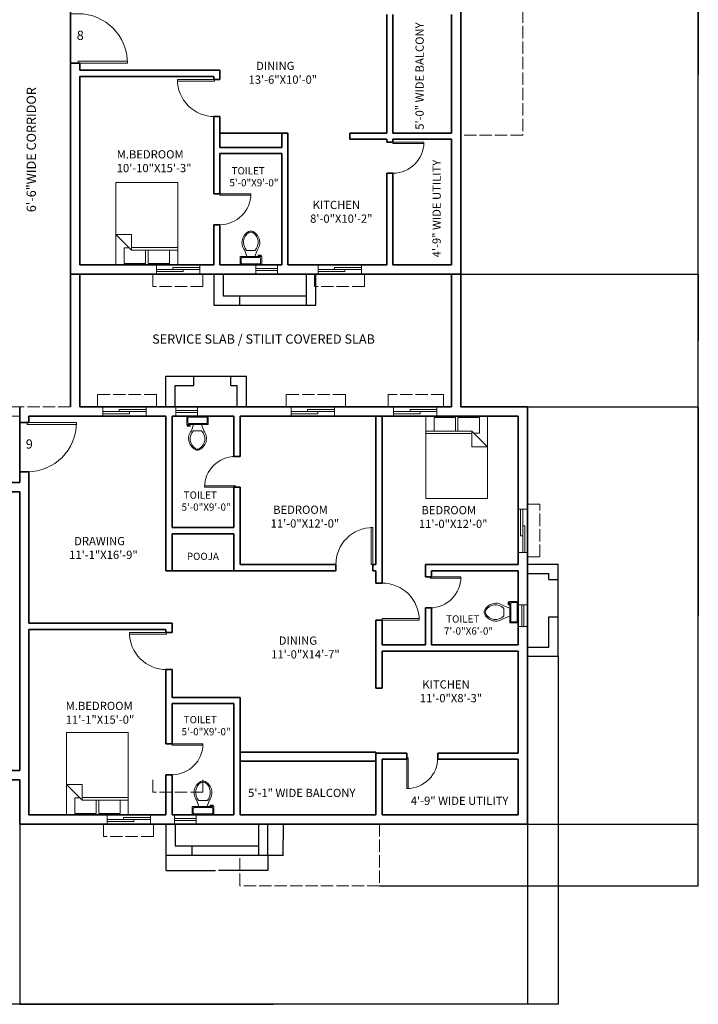
# Model space of a CAD drawing. Units: inches. Extents: x -69 to 2453, y 4803 to 7122.
# Tile 6 of 9: x 1794 to 2453, y 4803 to 5759. Entities that reach past the tile are written whole.
import ezdxf

# ---------------------------------------------------------------- set-up
doc = ezdxf.new("R2010")
doc.units = ezdxf.units.IN
doc.linetypes.add('ACAD_ISO02W100', pattern=[15, 12, -3])
for name, color, linetype, lineweight in [('A-ANNO-DIMS', 2, 'Continuous', 18), ('A-ANNO-IDEN', 2, 'Continuous', 18), ('A-AREA-IDEN', 7, 'Continuous', 18), ('A-DOOR', 3, 'Continuous', 18), ('A-FLOR-FIXT', 9, 'Continuous', 18), ('A-FLOR-OVHD', 8, 'ACAD_ISO02W100', 13), ('A-FURN', 8, 'Continuous', 18), ('A-GLAZ', 244, 'Continuous', 18), ('A-WALL', 7, 'Continuous', 35), ('A-WALL-SRVC', 7, 'Continuous', 30)]:
    doc.layers.add(name, color=color, linetype=linetype, lineweight=lineweight)
doc.styles.get("Standard").update_dxf_attribs({"font": 'arial.ttf'})
doc.dimstyles.get("Standard").update_dxf_attribs({"dimtxt": 0.18, "dimasz": 0.18, "dimexe": 0.18, "dimexo": 0.0625, "dimgap": 0.09, "dimtad": 0, "dimtih": 1, "dimtoh": 1, "dimdec": 4, "dimzin": 0, "dimdsep": 46, "dimtxsty": 'Standard', "dimcen": 0.09, "dimadec": 0, "dimazin": 0, "dimtfac": 1, "dimtdec": 4, "dimtofl": 0, "dimtmove": 0, "dimatfit": 3, "dimfxl": 1, "dimtolj": 1, "dimtzin": 0, "dimarcsym": 0})

# ---------------------------------------------------------------- blocks, each defined once
blk = doc.blocks.new('*U12')
for p, q in [((-40, 0), (-40, -6)), ((0, 0), (0, -6))]:
    blk.add_line(p, q)
blk.add_lwpolyline([(0, 0), (0, 40), (-1.75, 40), (-1.75, 0)], close=True)
blk.add_arc((0, 0), 40, 90, 180)
blk = doc.blocks.new('*U20')
for p, q in [((0, 0), (0, -6)), ((40, 0), (40, -6))]:
    blk.add_line(p, q)
blk.add_lwpolyline([(0, 0), (0, 40), (1.75, 40), (1.75, 0)], close=True)
blk.add_arc((0, 0), 40, 0, 90)
blk = doc.blocks.new('*U13')
for p, q in [((0, 0), (0, -6)), ((40, 0), (40, -6))]:
    blk.add_line(p, q)
blk.add_lwpolyline([(0, 0), (0, 40), (1.75, 40), (1.75, 0)], close=True)
blk.add_arc((0, 0), 40, 0, 90)
blk = doc.blocks.new('*U11')
for p, q in [((-40, 0), (-40, 6)), ((0, 0), (0, 6))]:
    blk.add_line(p, q)
blk.add_lwpolyline([(0, 0), (0, -40), (-1.75, -40), (-1.75, 0)], close=True)
blk.add_arc((0, 0), 40, 180, 270)
blk = doc.blocks.new('*U17')
for p, q in [((0, 0), (0, 6)), ((40, 0), (40, 6))]:
    blk.add_line(p, q)
blk.add_lwpolyline([(0, 0), (0, -40), (1.75, -40), (1.75, 0)], close=True)
blk.add_arc((0, 0), 40, 270, 0)
blk = doc.blocks.new('*U18')
for p, q in [((0, 0), (0, -6)), ((-40, 0), (-40, -6))]:
    blk.add_line(p, q)
blk.add_lwpolyline([(0, 0), (0, 40), (-1.75, 40), (-1.75, 0)], close=True)
blk.add_arc((0, 0), 40, 90, 180)
blk = doc.blocks.new('*U19')
for p, q in [((0, 0), (0, -6)), ((-40, 0), (-40, -6))]:
    blk.add_line(p, q)
blk.add_lwpolyline([(0, 0), (0, 40), (-1.75, 40), (-1.75, 0)], close=True)
blk.add_arc((0, 0), 40, 90, 180)
blk = doc.blocks.new('*U14')
for p, q in [((0, 0), (0, -6)), ((-40, 0), (-40, -6))]:
    blk.add_line(p, q)
blk.add_lwpolyline([(0, 0), (0, 40), (-1.75, 40), (-1.75, 0)], close=True)
blk.add_arc((0, 0), 40, 90, 180)
blk = doc.blocks.new('Bed - Queen')
for p, q in [((0, -80.00003), (0, 0)), ((0, 0), (59.99999, 0)), ((59.99999, 0), (59.99999, -80.00003)), ((7.99999, -1.2), (28.79998, -1.2)), ((7.99999, -14.4), (7.99999, -1.2)), ((28.79998, -1.2), (28.79998, -14.4)), ((31.19999, -1.2), (51.99999, -1.2)), ((31.19999, -14.4), (31.19999, -1.2)), ((51.99999, -1.2), (51.99999, -16.4)), ((0, -14.4), (44.8, -14.4)), ((44.8, -16.8), (0, -16.8)), ((59.99999, -29.6), (44.8, -14.4)), ((44.8, -14.4), (44.8, -29.6)), ((51.99999, -16.4), (46.79936, -16.4)), ((44.8, -29.6), (59.99999, -29.6)), ((59.99999, -80.00003), (0, -80.00003))]:
    blk.add_line(p, q)
blk = doc.blocks.new('*U33')
for p, q in [((-10, -8.5), (-8, -8.5)), ((-10, -9.5), (-10, -8.5)), ((-7, -9.5), (-10, -9.5)), ((-8, -8.5), (-8, -8)), ((-7, -8), (-7, -9.5)), ((-4, -8), (-6, -14)), ((4, -8), (6, -14)), ((9.5, -6), (9.5, -2)), ((4, -14), (-4, -14))]:
    blk.add_line(p, q)
blk.add_lwpolyline([(10.5, -8), (10.5, 0), (-10.5, 0), (-10.5, -8)], close=True)
for points in [[(-9.5, -2), (-9.5, -6)], [(8.5, -1), (-8.5, -1)], [(-8.5, -7), (8.5, -7)]]:
    blk.add_lwpolyline(points)
for centre, radius, start, end in [((-8.62, -1.88), 0.884, 81.8699, 188.1301), ((-8.62, -6.12), 0.884, 171.8699, 278.1301), ((8.62, -1.88), 0.884, 351.8699, 98.1301), ((8.62, -6.12), 0.884, 261.8699, 8.1301), ((3.52, -21.58), 12.17, 141.46911, 247.97143), ((4.2, -21.82), 11.33, 136.36773, 238.94682), ((-3.52, -21.58), 12.17, 292.02843, 38.53071), ((-4.2, -21.82), 11.33, 301.05301, 43.63209), ((0, -27.88), 4, 245.73182, 294.26817), ((0, -29), 4, 254.86053, 285.13947)]:
    blk.add_arc(centre, radius, start, end)
blk = doc.blocks.new('WINDOW-VENT-21IN')
for p, q in [((0, 5.5), (21, 5.5)), ((0, 3.5), (21, 3.5))]:
    blk.add_line(p, q)
blk.add_lwpolyline([(0, 9), (21, 9), (21, 0), (0, 0)], close=True)
blk = doc.blocks.new('WINDOW-SLIDING-42IN')
for p, q in [((2.5, 42), (2.5, 16)), ((4.5, 42), (4.5, 0)), ((4.5, 26), (6.5, 26)), ((6.5, 26), (6.5, 0)), ((4.5, 16), (2.5, 16))]:
    blk.add_line(p, q)
blk.add_lwpolyline([(0, 42), (9, 42), (9, 0), (0, 0)], close=True)
blk = doc.blocks.new('SUNSHADE-48IN')
for p, q in [((0, 0), (0, 12)), ((48.4, 12), (48.4, 0)), ((48.4, 0), (0, 0))]:
    blk.add_line(p, q)
blk = doc.blocks.new('SUNSHADE-57IN')
for p, q in [((57.14, 12), (0, 12)), ((0, 12), (0, 0)), ((57.14, 0), (57.14, 12))]:
    blk.add_line(p, q)
blk = doc.blocks.new('SUNSHADE-51IN')
for p, q in [((12, 51.36), (0, 51.36)), ((12, 0), (12, 51.36)), ((0, 0), (12, 0))]:
    blk.add_line(p, q)
blk = doc.blocks.new('SERVICE-BAY-78IN')
for p, q in [((0, 30), (78.14, 30)), ((0, 0), (0, 30)), ((27.07, 21), (27.07, 30)), ((63.07, 21), (63.07, 30)), ((78.14, 0), (78.14, 30)), ((9, 0), (9, 21)), ((9, 21), (27.07, 21)), ((63.07, 21), (69.14, 21)), ((69.14, 0), (69.14, 21))]:
    blk.add_line(p, q)
blk = doc.blocks.new('SERVICE-BAY-99IN')
for p, q in [((0, 30), (0, 0)), ((9, 30), (9, 9)), ((90.11, 0), (90.11, 30)), ((99.11, 0), (99.11, 30)), ((0, 0), (99.11, 0)), ((9, 9), (90.11, 9)), ((25.44, 0), (25.44, 9))]:
    blk.add_line(p, q)
blk = doc.blocks.new('*D67')
at = {"layer": 'A-ANNO-DIMS', "color": 0, "lineweight": -2, "transparency": 16777216}
for p, q in [((1935.51, 4947.65), (1935.51, 4932.67)), ((2034.62, 4947.65), (2034.62, 4932.67)), ((1935.69, 4932.85), (1983.66, 4932.85)), ((2034.44, 4932.85), (1986.47, 4932.85))]:
    blk.add_line(p, q, dxfattribs=at)
at = {"layer": 'A-ANNO-DIMS', "color": 0, "transparency": 16777216}
for points in [[(1935.69, 4932.88), (1935.69, 4932.82), (1935.51, 4932.85)], [(2034.44, 4932.88), (2034.44, 4932.82), (2034.62, 4932.85)]]:
    blk.add_solid(points, dxfattribs=at)
at = {"layer": 'Defpoints', "color": 0, "transparency": 16777216}
for p in [(1935.51, 4947.72), (2034.62, 4947.72), (2034.62, 4932.85)]:
    blk.add_point(p, dxfattribs=at)
at = {"layer": 'A-ANNO-DIMS', "color": 0, "transparency": 16777216, "insert": (1985.06, 4932.85), "char_height": 0.18, "attachment_point": 5}
blk.add_mtext('\\A1;SERVICE BAY 99 TYP.', dxfattribs=at)
blk = doc.blocks.new('*D68')
at = {"layer": 'A-ANNO-DIMS', "color": 0, "lineweight": -2, "transparency": 16777216}
for p, q in [((2034.68, 4977.72), (2049.67, 4977.72)), ((2049.49, 4977.54), (2049.49, 4962.9)), ((2049.49, 4947.9), (2049.49, 4962.53)), ((2034.68, 4947.72), (2049.67, 4947.72))]:
    blk.add_line(p, q, dxfattribs=at)
at = {"layer": 'A-ANNO-DIMS', "color": 0, "transparency": 16777216}
for points in [[(2049.46, 4977.54), (2049.52, 4977.54), (2049.49, 4977.72)], [(2049.46, 4947.9), (2049.52, 4947.9), (2049.49, 4947.72)]]:
    blk.add_solid(points, dxfattribs=at)
at = {"layer": 'Defpoints', "color": 0, "transparency": 16777216}
for p in [(2034.62, 4977.72), (2049.49, 4977.72), (2034.62, 4947.72)]:
    blk.add_point(p, dxfattribs=at)
at = {"layer": 'A-ANNO-DIMS', "color": 0, "transparency": 16777216, "insert": (2049.49, 4962.72), "char_height": 0.18, "attachment_point": 5}
blk.add_mtext('\\A1;30 TYP.', dxfattribs=at)
blk = doc.blocks.new('*D86')
at = {"layer": 'A-ANNO-DIMS', "color": 0, "lineweight": -2, "transparency": 16777216}
for p, q in [((1673.51, 5020.65), (1673.51, 4802.79)), ((1793.51, 5020.65), (1793.51, 4802.79)), ((1673.69, 4802.97), (1733.23, 4802.97)), ((1793.33, 4802.97), (1733.79, 4802.97))]:
    blk.add_line(p, q, dxfattribs=at)
at = {"layer": 'A-ANNO-DIMS', "color": 0, "transparency": 16777216}
for points in [[(1673.69, 4803), (1673.69, 4802.94), (1673.51, 4802.97)], [(1793.33, 4803), (1793.33, 4802.94), (1793.51, 4802.97)]]:
    blk.add_solid(points, dxfattribs=at)
at = {"layer": 'Defpoints', "color": 0, "transparency": 16777216}
for p in [(1673.51, 5020.72), (1793.51, 5020.72), (1793.51, 4802.97)]:
    blk.add_point(p, dxfattribs=at)
at = {"layer": 'A-ANNO-DIMS', "color": 0, "transparency": 16777216, "insert": (1733.51, 4802.97), "char_height": 0.18, "attachment_point": 5}
blk.add_mtext('\\A1;120', dxfattribs=at)
blk = doc.blocks.new('*D87')
at = {"layer": 'A-ANNO-DIMS', "color": 0, "lineweight": -2, "transparency": 16777216}
for p, q in [((1793.51, 4977.65), (1793.51, 4802.79)), ((2286.51, 4977.65), (2286.51, 4802.79)), ((1793.69, 4802.97), (2039.72, 4802.97)), ((2286.33, 4802.97), (2040.3, 4802.97))]:
    blk.add_line(p, q, dxfattribs=at)
at = {"layer": 'A-ANNO-DIMS', "color": 0, "transparency": 16777216}
for points in [[(1793.69, 4803), (1793.69, 4802.94), (1793.51, 4802.97)], [(2286.33, 4803), (2286.33, 4802.94), (2286.51, 4802.97)]]:
    blk.add_solid(points, dxfattribs=at)
at = {"layer": 'Defpoints', "color": 0, "transparency": 16777216}
for p in [(1793.51, 4977.72), (2286.51, 4977.72), (2286.51, 4802.97)]:
    blk.add_point(p, dxfattribs=at)
at = {"layer": 'A-ANNO-DIMS', "color": 0, "transparency": 16777216, "insert": (2040.01, 4802.97), "char_height": 0.18, "attachment_point": 5}
blk.add_mtext('\\A1;493', dxfattribs=at)
blk = doc.blocks.new('*D88')
at = {"layer": 'A-ANNO-DIMS', "color": 0, "lineweight": -2, "transparency": 16777216}
for p, q in [((2286.57, 5382.72), (2452.44, 5382.72)), ((2452.26, 5382.54), (2452.26, 5180.4)), ((2452.26, 4977.9), (2452.26, 5180.03)), ((2286.57, 4977.72), (2452.44, 4977.72))]:
    blk.add_line(p, q, dxfattribs=at)
at = {"layer": 'A-ANNO-DIMS', "color": 0, "transparency": 16777216}
for points in [[(2452.23, 5382.54), (2452.29, 5382.54), (2452.26, 5382.72)], [(2452.23, 4977.9), (2452.29, 4977.9), (2452.26, 4977.72)]]:
    blk.add_solid(points, dxfattribs=at)
at = {"layer": 'Defpoints', "color": 0, "transparency": 16777216}
for p in [(2286.51, 5382.72), (2452.26, 5382.72), (2286.51, 4977.72)]:
    blk.add_point(p, dxfattribs=at)
at = {"layer": 'A-ANNO-DIMS', "color": 0, "transparency": 16777216, "insert": (2452.26, 5180.22), "char_height": 0.18, "attachment_point": 5}
blk.add_mtext('\\A1;405', dxfattribs=at)
blk = doc.blocks.new('*D89')
at = {"layer": 'A-ANNO-DIMS', "color": 0, "lineweight": -2, "transparency": 16777216}
for p, q in [((2222.07, 5511.72), (2452.44, 5511.72)), ((2452.26, 5511.54), (2452.26, 5447.4)), ((2452.26, 5382.9), (2452.26, 5447.03)), ((2222.07, 5382.72), (2452.44, 5382.72))]:
    blk.add_line(p, q, dxfattribs=at)
at = {"layer": 'A-ANNO-DIMS', "color": 0, "transparency": 16777216}
for points in [[(2452.23, 5511.54), (2452.29, 5511.54), (2452.26, 5511.72)], [(2452.23, 5382.9), (2452.29, 5382.9), (2452.26, 5382.72)]]:
    blk.add_solid(points, dxfattribs=at)
at = {"layer": 'Defpoints', "color": 0, "transparency": 16777216}
for p in [(2222.01, 5511.72), (2452.26, 5511.72), (2222.01, 5382.72)]:
    blk.add_point(p, dxfattribs=at)
at = {"layer": 'A-ANNO-DIMS', "color": 0, "transparency": 16777216, "insert": (2452.26, 5447.22), "char_height": 0.18, "attachment_point": 5}
blk.add_mtext('\\A1;129', dxfattribs=at)
blk = doc.blocks.new('*D90')
at = {"layer": 'A-ANNO-DIMS', "color": 0, "lineweight": -2, "transparency": 16777216}
for p, q in [((2222.07, 5898.72), (2452.44, 5898.72)), ((2452.26, 5898.54), (2452.26, 5705.4)), ((2452.26, 5511.9), (2452.26, 5705.03)), ((2222.07, 5511.72), (2452.44, 5511.72))]:
    blk.add_line(p, q, dxfattribs=at)
at = {"layer": 'A-ANNO-DIMS', "color": 0, "transparency": 16777216}
for points in [[(2452.23, 5898.54), (2452.29, 5898.54), (2452.26, 5898.72)], [(2452.23, 5511.9), (2452.29, 5511.9), (2452.26, 5511.72)]]:
    blk.add_solid(points, dxfattribs=at)
at = {"layer": 'Defpoints', "color": 0, "transparency": 16777216}
for p in [(2222.01, 5898.72), (2452.26, 5898.72), (2222.01, 5511.72)]:
    blk.add_point(p, dxfattribs=at)
at = {"layer": 'A-ANNO-DIMS', "color": 0, "transparency": 16777216, "insert": (2452.26, 5705.22), "char_height": 0.18, "attachment_point": 5}
blk.add_mtext('\\A1;387', dxfattribs=at)
blk = doc.blocks.new('*D95')
at = {"layer": 'A-ANNO-DIMS', "color": 0, "lineweight": -2, "transparency": 16777216}
for p, q in [((96.509262, 5020.652777), (96.509262, 4802.785277)), ((2286.509262, 4977.652777), (2286.509262, 4802.785277)), ((96.689262, 4802.965277), (1191.149262, 4802.965277)), ((2286.329262, 4802.965277), (1191.869262, 4802.965277))]:
    blk.add_line(p, q, dxfattribs=at)
at = {"layer": 'A-ANNO-DIMS', "color": 0, "transparency": 16777216}
for points in [[(96.689262, 4802.995277), (96.689262, 4802.935277), (96.509262, 4802.965277)], [(2286.329262, 4802.995277), (2286.329262, 4802.935277), (2286.509262, 4802.965277)]]:
    blk.add_solid(points, dxfattribs=at)
at = {"layer": 'Defpoints', "color": 0, "transparency": 16777216}
for p in [(96.509262, 5020.715277), (2286.509262, 4977.715277), (2286.509262, 4802.965277)]:
    blk.add_point(p, dxfattribs=at)
at = {"layer": 'A-ANNO-DIMS', "color": 0, "transparency": 16777216, "insert": (1191.509262, 4802.965277), "char_height": 0.18, "attachment_point": 5}
blk.add_mtext('\\A1;2190', dxfattribs=at)
blk = doc.blocks.new('*D96')
at = {"layer": 'A-ANNO-DIMS', "color": 0, "lineweight": -2, "transparency": 16777216}
for p, q in [((2044.63, 7006.72), (2452.44, 7006.72)), ((2452.26, 7006.54), (2452.26, 5962.4)), ((2452.26, 4917.9), (2452.26, 5962.03)), ((2143.12, 4917.72), (2452.44, 4917.72))]:
    blk.add_line(p, q, dxfattribs=at)
at = {"layer": 'A-ANNO-DIMS', "color": 0, "transparency": 16777216}
for points in [[(2452.23, 7006.54), (2452.29, 7006.54), (2452.26, 7006.72)], [(2452.23, 4917.9), (2452.29, 4917.9), (2452.26, 4917.72)]]:
    blk.add_solid(points, dxfattribs=at)
at = {"layer": 'Defpoints', "color": 0, "transparency": 16777216}
for p in [(2044.57, 7006.72), (2452.26, 7006.72), (2143.06, 4917.72)]:
    blk.add_point(p, dxfattribs=at)
at = {"layer": 'A-ANNO-DIMS', "color": 0, "transparency": 16777216, "insert": (2452.26, 5962.22), "char_height": 0.18, "attachment_point": 5}
blk.add_mtext('\\A1;2089', dxfattribs=at)
blk = doc.blocks.new('*D105')
at = {"layer": 'A-ANNO-DIMS', "color": 0, "lineweight": -2, "transparency": 16777216}
for p, q in [((66.509262, 5170.610035), (66.509262, 4802.785277)), ((2316.509262, 5140.587945), (2316.509262, 4802.785277)), ((66.689262, 4802.965277), (1191.149262, 4802.965277)), ((2316.329262, 4802.965277), (1191.869262, 4802.965277))]:
    blk.add_line(p, q, dxfattribs=at)
at = {"layer": 'A-ANNO-DIMS', "color": 0, "transparency": 16777216}
for points in [[(66.689262, 4802.995277), (66.689262, 4802.935277), (66.509262, 4802.965277)], [(2316.329262, 4802.995277), (2316.329262, 4802.935277), (2316.509262, 4802.965277)]]:
    blk.add_solid(points, dxfattribs=at)
at = {"layer": 'Defpoints', "color": 0, "transparency": 16777216}
for p in [(66.509262, 5170.672535), (2316.509262, 5140.650445), (2316.509262, 4802.965277)]:
    blk.add_point(p, dxfattribs=at)
at = {"layer": 'A-ANNO-DIMS', "color": 0, "transparency": 16777216, "insert": (1191.509262, 4802.965277), "char_height": 0.18, "attachment_point": 5}
blk.add_mtext('\\A1;2250', dxfattribs=at)

msp = doc.modelspace()

# ---------------------------------------------------------------- linework, layer by layer
at = {"layer": 'A-FLOR-OVHD'}
for p, q in [((2282.01, 5767.63), (2282.01, 5646.75)), ((2282.01, 5646.75), (2222.01, 5646.75)), ((2109.75, 5394.72), (2052.22, 5394.72)), ((2052.22, 5394.72), (2052.22, 5382.72)), ((2109.75, 5382.72), (2109.75, 5394.72)), ((2204.95, 5394.72), (2151.19, 5394.72)), ((2151.19, 5394.72), (2151.19, 5382.72)), ((2204.95, 5382.72), (2204.95, 5394.72)), ((1843.01, 5382.72), (1673.51, 5382.72)), ((1793.51, 5373.72), (1673.51, 5373.72)), ((2143.06, 4977.72), (2143.06, 4917.72)), ((2007.19, 4917.72), (2007.19, 4947.72)), ((2143.06, 4917.72), (2007.19, 4917.72))]:
    msp.add_line(p, q, dxfattribs=at)
at = {"layer": 'A-WALL'}
for p, q in [((2222.01, 6543.72), (2222.01, 5382.72)), ((1843.01, 6308.22), (1843.01, 5382.72)), ((2150.01, 5763.72), (2150.01, 5648.72)), ((2156.01, 5763.72), (2156.01, 5648.72)), ((2213.01, 5763.72), (2213.01, 5648.72)), ((1852.01, 5716.52), (1843.01, 5716.52)), ((1852.01, 5716.52), (1852.01, 5709.72)), ((1852.01, 5709.72), (1988.01, 5709.72)), ((1988.01, 5709.72), (1988.01, 5700.72)), ((1852.01, 5703.72), (1982.01, 5703.72)), ((1852.01, 5703.72), (1852.01, 5520.72)), ((1982.01, 5703.72), (1982.01, 5700.72)), ((1982.01, 5700.72), (1988.01, 5700.72)), ((1982.01, 5664.72), (1988.01, 5664.72)), ((1982.01, 5664.72), (1982.01, 5589.72)), ((1988.01, 5664.72), (1988.01, 5634.72)), ((1988.01, 5648.72), (2054.01, 5648.72)), ((2048.01, 5648.72), (2048.01, 5634.72)), ((2054.01, 5648.72), (2054.01, 5520.72)), ((2114.01, 5648.72), (2114.01, 5642.72)), ((2114.01, 5648.72), (2150.01, 5648.72)), ((2150.01, 5642.72), (2114.01, 5642.72)), ((2150.01, 5642.72), (2150.01, 5639.72)), ((2156.01, 5648.72), (2213.01, 5648.72)), ((2156.01, 5642.72), (2156.01, 5639.72)), ((2156.01, 5642.72), (2213.01, 5642.72)), ((2213.01, 5642.72), (2213.01, 5520.72)), ((1988.01, 5634.72), (2048.01, 5634.72)), ((2150.01, 5639.72), (2156.01, 5639.72)), ((1988.01, 5628.72), (2048.01, 5628.72)), ((1988.01, 5628.72), (1988.01, 5589.72)), ((2048.01, 5628.72), (2048.01, 5520.72)), ((2150.01, 5609.72), (2156.01, 5609.72)), ((2150.01, 5609.72), (2150.01, 5520.72)), ((2156.01, 5609.72), (2156.01, 5520.72)), ((1988.01, 5589.72), (1982.01, 5589.72)), ((1988.01, 5559.72), (1982.01, 5559.72)), ((1982.01, 5559.72), (1982.01, 5520.72)), ((1988.01, 5559.72), (1988.01, 5520.72)), ((1852.01, 5520.72), (1982.01, 5520.72)), ((1988.01, 5520.72), (2048.01, 5520.72)), ((2054.01, 5520.72), (2150.01, 5520.72)), ((2156.01, 5520.72), (2213.01, 5520.72)), ((1843.01, 5511.72), (2222.01, 5511.72)), ((1852.01, 5511.72), (1852.01, 5382.72)), ((2213.01, 5511.72), (2213.01, 5382.72)), ((1793.51, 5382.72), (1793.51, 5309.33)), ((1852.01, 5382.72), (2213.01, 5382.72)), ((2222.01, 5382.72), (2286.51, 5382.72)), ((2286.51, 5382.72), (2286.51, 4977.72)), ((1802.51, 5373.72), (1935.51, 5373.72)), ((1802.51, 5373.72), (1802.51, 5367.72)), ((1935.51, 5373.72), (1935.51, 5223.72)), ((1941.51, 5373.72), (1941.51, 5265.72)), ((1941.51, 5373.72), (2001.51, 5373.72)), ((2001.51, 5373.72), (2001.51, 5334.72)), ((2007.51, 5373.72), (2007.51, 5334.72)), ((2007.51, 5373.72), (2277.51, 5373.72)), ((2139.51, 5373.72), (2139.51, 5229.72)), ((2145.51, 5373.72), (2145.51, 5211.72)), ((2277.51, 5373.72), (2277.51, 5229.72)), ((1802.51, 5367.72), (1793.51, 5367.72)), ((2001.51, 5334.72), (2007.51, 5334.72)), ((1802.51, 5319.72), (1793.51, 5319.72)), ((1802.51, 5319.72), (1802.51, 5172.72)), ((1673.51, 5309.33), (1793.51, 5309.33)), ((1673.51, 5300.33), (1793.51, 5300.33)), ((1793.51, 5300.33), (1793.51, 5029.72)), ((2001.51, 5304.72), (2007.51, 5304.72)), ((2001.51, 5304.72), (2001.51, 5265.72)), ((2007.51, 5304.72), (2007.51, 5229.72)), ((1941.51, 5265.72), (2001.51, 5265.72)), ((1941.51, 5259.72), (2001.51, 5259.72)), ((1941.51, 5259.72), (1941.51, 5223.72)), ((2001.51, 5259.72), (2001.51, 5223.72)), ((2007.51, 5229.72), (2100.51, 5229.72)), ((2100.51, 5223.72), (2100.51, 5229.72)), ((2136.51, 5223.72), (2136.51, 5229.72)), ((2136.51, 5229.72), (2139.51, 5229.72)), ((2187.51, 5229.72), (2277.51, 5229.72)), ((2187.51, 5229.72), (2187.51, 5217.72)), ((1935.51, 5223.72), (2100.51, 5223.72)), ((2136.51, 5223.72), (2139.51, 5223.72)), ((2139.51, 5223.72), (2139.51, 5211.72)), ((2193.51, 5223.72), (2277.51, 5223.72)), ((2193.51, 5223.72), (2193.51, 5217.72)), ((2277.51, 5223.72), (2277.51, 5151.72)), ((2145.51, 5211.72), (2139.51, 5211.72)), ((2193.51, 5217.72), (2187.51, 5217.72)), ((2193.51, 5187.72), (2187.51, 5187.72)), ((2187.51, 5187.72), (2187.51, 5151.72)), ((2193.51, 5187.72), (2193.51, 5151.72)), ((1802.51, 5172.72), (1941.51, 5172.72)), ((1941.51, 5172.72), (1941.51, 5163.72)), ((2145.51, 5175.72), (2139.51, 5175.72)), ((2139.51, 5175.72), (2139.51, 5109.72)), ((2145.51, 5175.72), (2145.51, 5151.72)), ((1802.51, 5166.72), (1935.51, 5166.72)), ((1802.51, 5166.72), (1802.51, 4986.72)), ((1935.51, 5166.72), (1935.51, 5163.72)), ((1935.51, 5163.72), (1941.51, 5163.72)), ((2145.51, 5151.72), (2187.51, 5151.72)), ((2145.51, 5145.72), (2277.51, 5145.72)), ((2145.51, 5145.72), (2145.51, 5109.72)), ((2193.51, 5151.72), (2277.51, 5151.72)), ((2277.51, 5145.72), (2277.51, 5046.72)), ((1935.51, 5127.72), (1941.51, 5127.72)), ((1935.51, 5127.72), (1935.51, 5055.72)), ((1941.51, 5127.72), (1941.51, 5100.72)), ((2139.51, 5109.72), (2145.51, 5109.72)), ((1941.51, 5100.72), (2007.51, 5100.72)), ((2007.51, 5100.72), (2007.51, 4986.72)), ((1941.51, 5094.72), (2001.51, 5094.72)), ((1941.51, 5094.72), (1941.51, 5055.72)), ((2001.51, 5094.72), (2001.51, 4986.72)), ((1941.51, 5055.72), (1935.51, 5055.72)), ((2007.51, 5047.72), (2139.51, 5047.72)), ((2139.51, 5047.72), (2139.51, 4986.72)), ((2007.51, 5038.72), (2139.51, 5038.72)), ((2139.51, 5046.72), (2169.51, 5046.72)), ((2145.51, 5040.72), (2169.51, 5040.72)), ((2145.51, 5040.72), (2145.51, 4986.72)), ((2169.51, 5040.72), (2169.51, 5046.72)), ((2199.51, 5040.72), (2199.51, 5046.72)), ((2199.51, 5046.72), (2277.51, 5046.72)), ((2199.51, 5040.72), (2277.51, 5040.72)), ((2277.51, 5040.72), (2277.51, 4986.72)), ((1673.51, 5029.72), (1793.51, 5029.72)), ((354.66, 5020.72), (1793.51, 5020.72)), ((1793.51, 5020.72), (1793.51, 4977.72)), ((1941.51, 5025.72), (1935.51, 5025.72)), ((1935.51, 5025.72), (1935.51, 4986.72)), ((1941.51, 5025.72), (1941.51, 4986.72)), ((1802.51, 4986.72), (1935.51, 4986.72)), ((1941.51, 4986.72), (2001.51, 4986.72)), ((2007.51, 4986.72), (2139.51, 4986.72)), ((2145.51, 4986.72), (2277.51, 4986.72)), ((1793.51, 4977.72), (2286.51, 4977.72))]:
    msp.add_line(p, q, dxfattribs=at)
at = {"layer": 'A-WALL-SRVC'}
for p, q in [((2286.51, 5230.2), (2316.51, 5230.2)), ((2316.51, 5140.65), (2316.51, 5230.2)), ((2286.51, 5221.2), (2307.51, 5221.2)), ((2307.51, 5215.13), (2307.51, 5221.2)), ((2307.51, 5215.13), (2316.51, 5215.13)), ((2307.51, 5149.65), (2307.51, 5179.13)), ((2307.51, 5179.13), (2316.51, 5179.13)), ((2286.51, 5149.65), (2307.51, 5149.65)), ((2286.51, 5140.65), (2316.51, 5140.65))]:
    msp.add_line(p, q, dxfattribs=at)

# ---------------------------------------------------------------- block references
at = {"layer": 'A-DOOR'}
for name, p, xscale, yscale, zscale, rotation in [('*U12', (1850.21, 5716.52), 1.199999999999977, 1.199999999999977, 1.199999999999977, 270.0000000000001), ('*U17', (1982.61, 5700.72), 0.9, 0.9, 0.9, 270), ('*U13', (2156.01, 5639.72), 0.75, 0.75, 0.75, 270.0000000000001), ('*U13', (1988.01, 5589.72), 0.75, 0.75, 0.75, 270.0000000000001), ('*U20', (1800.71, 5367.72), 1.199999999999977, 1.199999999999977, 1.199999999999977, 270.0000000000001), ('*U11', (2003.01, 5304.72), 0.75, 0.75, 0.75, 270.0000000000001), ('*U18', (2145.51, 5175.72), 0.9, 0.9, 0.9, 270), ('*U13', (2192.01, 5217.72), 0.75, 0.75, 0.75, 270.0000000000001), ('*U17', (1936.11, 5163.72), 0.9, 0.9, 0.9, 270), ('*U13', (1941.51, 5055.72), 0.75, 0.75, 0.75, 270.0000000000001), ('*U14', (2169.51, 5042.22), 0.75, 0.75, 0.75, 180)]:
    msp.add_blockref(name, p, dxfattribs=dict(at, xscale=xscale, yscale=yscale, zscale=zscale, rotation=rotation))
at = {"layer": 'A-DOOR', "xscale": 0.9, "yscale": 0.9, "zscale": 0.9}
msp.add_blockref('*U19', (2136.51, 5229.72), dxfattribs=at)
at = {"layer": 'A-FLOR-FIXT'}
for p, rotation in [((2018.01, 5520.72), 180), ((2277.51, 5183.51), 270), ((1971.51, 4986.72), 180)]:
    msp.add_blockref('*U33', p, dxfattribs=dict(at, rotation=rotation))
msp.add_blockref('*U33', (1966.2, 5373.72), dxfattribs=at)
at = {"layer": 'A-FLOR-OVHD'}
for name, p in [('SUNSHADE-48IN', (1922.89, 5499.72)), ('SUNSHADE-48IN', (2079.86, 5499.72)), ('SUNSHADE-57IN', (1869.14, 5382.72)), ('SUNSHADE-51IN', (2286.51, 5237.15)), ('SUNSHADE-48IN', (1922.89, 5008.72)), ('SUNSHADE-48IN', (1874.98, 4965.72))]:
    msp.add_blockref(name, p, dxfattribs=at)
at = {"layer": 'A-FURN', "rotation": 180}
for p in [(1947.01, 5520.72), (1899.01, 4986.72)]:
    msp.add_blockref('Bed - Queen', p, dxfattribs=at)
at = {"layer": 'A-FURN'}
msp.add_blockref('Bed - Queen', (2187.88, 5373.72), dxfattribs=at)
at = {"layer": 'A-GLAZ'}
for name, p, rotation in [('WINDOW-SLIDING-42IN', (1926.34, 5520.72), 269.9999999999964), ('WINDOW-SLIDING-42IN', (2083.31, 5520.72), 269.999999999996), ('WINDOW-SLIDING-42IN', (1874.23, 5382.72), 269.9999999999984), ('WINDOW-SLIDING-42IN', (2057.09, 5382.72), 270.0000000000029), ('WINDOW-SLIDING-42IN', (2156.56, 5382.72), 269.9999999999984), ('WINDOW-VENT-21IN', (2277.51, 5190.72), 270.0000000000005), ('WINDOW-SLIDING-42IN', (1878.44, 4986.72), 269.9999999999982)]:
    msp.add_blockref(name, p, dxfattribs=dict(at, rotation=rotation))
for name, p in [('WINDOW-VENT-21IN', (2022.94, 5511.72)), ('WINDOW-VENT-21IN', (1945.2, 5373.72)), ('WINDOW-SLIDING-42IN', (2277.51, 5241.48)), ('WINDOW-VENT-21IN', (1943.73, 4977.72))]:
    msp.add_blockref(name, p, dxfattribs=at)
at = {"layer": 'A-WALL-SRVC'}
for name, p in [('SERVICE-BAY-99IN', (1982.01, 5481.72)), ('SERVICE-BAY-78IN', (1935.51, 5382.72)), ('SERVICE-BAY-99IN', (1935.51, 4947.72))]:
    msp.add_blockref(name, p, dxfattribs=at)

# ---------------------------------------------------------------- texts
at = {"layer": 'A-ANNO-IDEN', "char_height": 8, "attachment_point": 1}
for s, insert in [('{\\H1.125x;8} ', (1848.93, 5748.07)), ('{\\H1.125x;9} ', (1799.43, 5351.27))]:
    msp.add_mtext_dynamic_manual_height_columns(s, width=10.4994, gutter_width=12.5, heights=[0], dxfattribs=dict(at, insert=insert))
at = {"layer": 'A-AREA-IDEN', "attachment_point": 1, "rotation": 90}
for s, width, insert, char_height in [('5\'-0" WIDE BALCONY', 114.3745, (2177.88, 5651.91), 8), ('6\'-6"WIDE CORRIDOR', 131.0566, (1800.26, 5571.82), 9), ('4\'-9" WIDE UTILITY', 99.5525, (2194.4, 5528.01), 8)]:
    msp.add_mtext_dynamic_manual_height_columns(s, width=width, gutter_width=12.5, heights=[0], dxfattribs=dict(at, insert=insert, char_height=char_height))
at = {"layer": 'A-AREA-IDEN', "attachment_point": 1}
for s, width, insert, char_height in [('   DINING\\P13\'-6"X10\'-0"', 63.2359, (2015.77, 5717.9), 8), ('M.BEDROOM\\P10\'-10"X15\'-3"', 69.6032, (1887.72, 5632.02), 8), (' TOILET\\P5\'-0"X9\'-0"', 45.2002, (1997.2, 5615.61), 7), (' KITCHEN\\P8\'-0"X10\'-2"', 58.1282, (2075.57, 5582.91), 8), ('SERVICE SLAB / STILIT COVERED SLAB', 244.2019, (1922.18, 5453.19), 9), (' TOILET\\P5\'-0"X9\'-0"', 45.2002, (1950.7, 5300.72), 7), (' BEDROOM\\P11\'-0"X12\'-0"', 64.9911, (2037.22, 5286.95), 8), (' BEDROOM\\P11\'-0"X12\'-0"', 64.9911, (2181.22, 5286.57), 8), ('  DRAWING\\P11\'-1"X16\'-9"', 66.0939, (1841.55, 5256.51), 8), ('POOJA', 33.9191, (1955.86, 5241.21), 7), (' TOILET\\P7\'-0"X6\'-0"', 45.2002, (2205.54, 5180.38), 7), ('   DINING\\P11\'-0"X14\'-7"', 63.2359, (2037.71, 5159.9), 8), (' KITCHEN\\P11\'-0"X8\'-3"', 58.1282, (2182.07, 5117.37), 8), ('M.BEDROOM\\P11\'-1"X15\'-0"', 69.6032, (1838.22, 5096.52), 8), (' TOILET\\P5\'-0"X9\'-0"', 45.2002, (1950.7, 5082.64), 7), ('5\'-1" WIDE BALCONY', 114.3745, (2015.32, 5012.03), 8), ('4\'-9" WIDE UTILITY', 99.5525, (2173.3, 5004.37), 8)]:
    msp.add_mtext_dynamic_manual_height_columns(s, width=width, gutter_width=12.5, heights=[0], dxfattribs=dict(at, insert=insert, char_height=char_height))

# ---------------------------------------------------------------- dimensions: what is measured, and where the dimension line sits
at = {"layer": 'A-ANNO-DIMS'}
for base, p1, p2, picture, middle in [((2452.26, 7006.72), (2143.06, 4917.72), (2044.57, 7006.72), '*D96', (2452.26, 5962.22)), ((2452.26, 5898.72), (2222.01, 5511.72), (2222.01, 5898.72), '*D90', (2452.26, 5705.22)), ((2452.26, 5511.72), (2222.01, 5382.72), (2222.01, 5511.72), '*D89', (2452.26, 5447.22)), ((2452.26, 5382.72), (2286.51, 4977.72), (2286.51, 5382.72), '*D88', (2452.26, 5180.22))]:
    dim = msp.add_linear_dim(base=base, p1=p1, p2=p2, angle=90, dimstyle='Standard', override={"dimdec": 0, "dimlfac": 1, "dimrnd": 0, "dimzin": 0, "dimdsep": 46, "dimlunit": 2}, dxfattribs=at)
    dim.commit()
    dim.dimension.update_dxf_attribs({"geometry": picture, "text_midpoint": middle})
for base, p1, p2, picture, middle in [((2316.51, 4802.97), (66.51, 5170.67), (2316.51, 5140.65), '*D105', (1191.51, 4802.97)), ((2286.51, 4802.97), (96.51, 5020.72), (2286.51, 4977.72), '*D95', (1191.51, 4802.97)), ((1793.51, 4802.97), (1673.51, 5020.72), (1793.51, 5020.72), '*D86', (1733.51, 4802.97)), ((2286.51, 4802.97), (1793.51, 4977.72), (2286.51, 4977.72), '*D87', (2040.01, 4802.97))]:
    dim = msp.add_linear_dim(base=base, p1=p1, p2=p2, dimstyle='Standard', override={"dimdec": 0, "dimlfac": 1, "dimrnd": 0, "dimzin": 0, "dimdsep": 46, "dimlunit": 2}, dxfattribs=at)
    dim.commit()
    dim.dimension.update_dxf_attribs({"geometry": picture, "text_midpoint": middle})
dim = msp.add_linear_dim(base=(2049.49, 4977.72), p1=(2034.62, 4947.72), p2=(2034.62, 4977.72), angle=90, text='<> TYP.', dimstyle='Standard', override={"dimdec": 0, "dimlfac": 1, "dimrnd": 0, "dimzin": 0, "dimdsep": 46, "dimlunit": 2}, dxfattribs=at)
dim.commit()
dim.dimension.update_dxf_attribs({"geometry": '*D68', "text_midpoint": (2049.49, 4962.72)})
dim = msp.add_linear_dim(base=(2034.62, 4932.85), p1=(1935.51, 4947.72), p2=(2034.62, 4947.72), text='SERVICE BAY <> TYP.', dimstyle='Standard', override={"dimdec": 0, "dimlfac": 1, "dimrnd": 0, "dimzin": 0, "dimdsep": 46, "dimlunit": 2}, dxfattribs=at)
dim.commit()
dim.dimension.update_dxf_attribs({"geometry": '*D67', "text_midpoint": (1985.06, 4932.85)})

doc.saveas('drawing.dxf')
